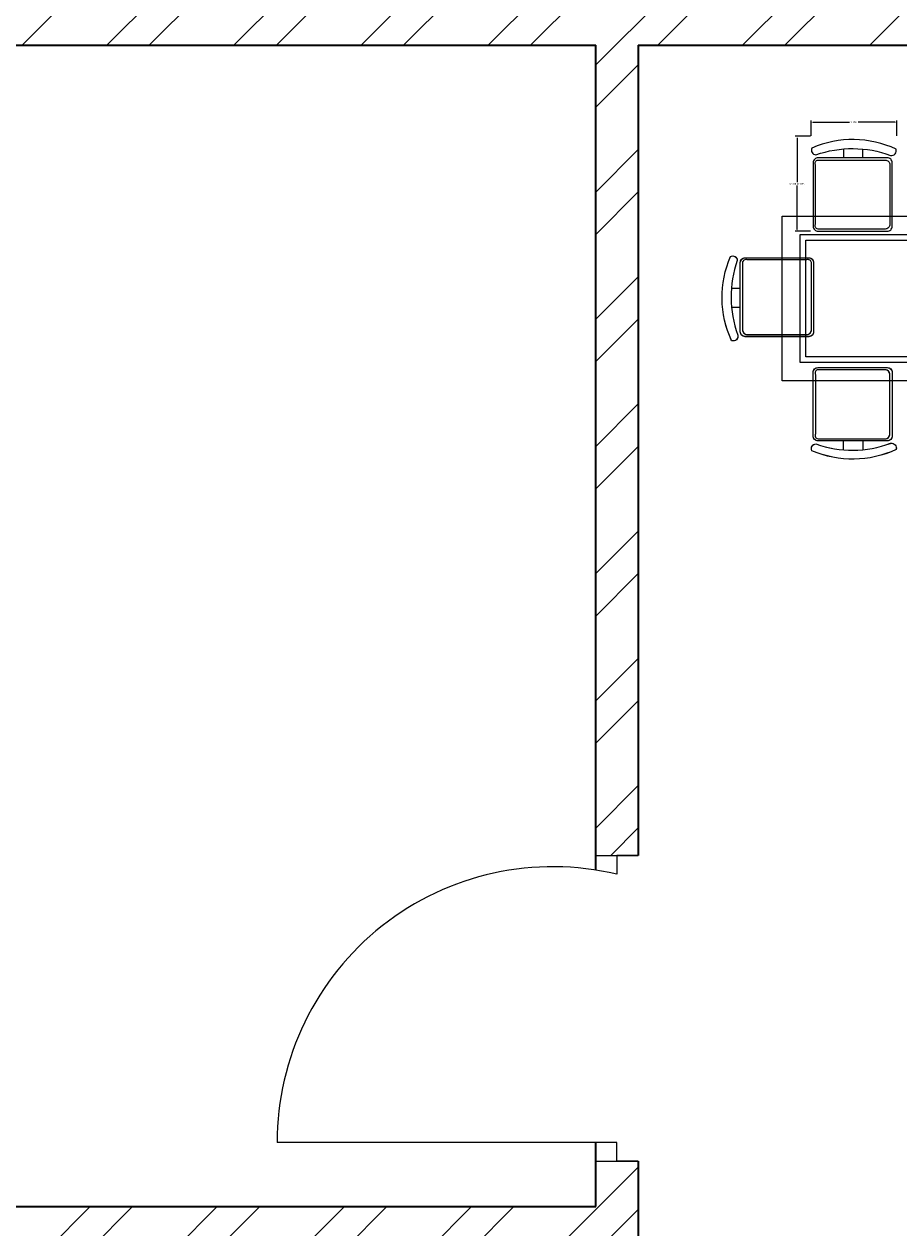
# Model space of a CAD drawing. Units: inches. Extents: x 2120 to 4013, y 1390 to 3019.
# Tile 6 of 59: x 2355 to 2448, y 1740 to 1868. Entities that reach past the tile are written whole.
import ezdxf

# ---------------------------------------------------------------- set-up
doc = ezdxf.new("R2010")
doc.units = ezdxf.units.IN
for name, color, linetype, lineweight in [('A-ANNO-DIMS', 2, 'Continuous', 18), ('A-DOOR', 3, 'Continuous', 18), ('A-FURN', 8, 'Continuous', 13), ('A-WALL', 7, 'Continuous', 35), ('A-WALL-PATT', 252, 'Continuous', 13)]:
    doc.layers.add(name, color=color, linetype=linetype, lineweight=lineweight)
doc.styles.get("Standard").update_dxf_attribs({"font": 'arial.ttf'})
doc.dimstyles.get("Standard").update_dxf_attribs({"dimtxt": 0.18, "dimasz": 0.18, "dimexe": 0.18, "dimexo": 0.0625, "dimgap": 0.09, "dimtad": 0, "dimtih": 1, "dimtoh": 1, "dimdec": 4, "dimzin": 0, "dimdsep": 46, "dimtxsty": 'Standard', "dimcen": 0.09, "dimadec": 0, "dimazin": 0, "dimtfac": 1, "dimtdec": 4, "dimtofl": 0, "dimtmove": 0, "dimatfit": 3, "dimfxl": 1, "dimtolj": 1, "dimtzin": 0, "dimarcsym": 0})

# ---------------------------------------------------------------- blocks, each defined once
blk = doc.blocks.new('DOOR-SWING-36IN-103p48DEG')
for p, q in [((33.75, 32.39), (38.25, 32.39)), ((38.25, 32.39), (36, 32.39)), ((36, 32.39), (36, 30.39)), ((36, 2), (0, 2)), ((36, 0), (36, 2)), ((33.75, 0), (38.25, 0)), ((38.25, 0), (36, 0))]:
    blk.add_line(p, q)
blk.add_arc((29.19, 2), 29.19, 76.5207, 180)
blk = doc.blocks.new('TABLE-DINING')
for points in [[(0, 17.41), (29.01, 17.41), (29.01, 0), (0, 0)], [(1.93, 15.47), (27.08, 15.47), (27.08, 1.93), (1.93, 1.93)], [(2.51, 14.89), (26.5, 14.89), (26.5, 2.51), (2.51, 2.51)]]:
    blk.add_lwpolyline(points, close=True)
blk = doc.blocks.new('CHAIR-DINING-07')
for points in [[(0.62, 8.03, -0.578392), (0.02, 8.69, -0.214524), (8.94, 8.81, -0.552014), (8.52, 8.09, 0.175809), (0.62, 8.03)], [(8.29, 7.77, -0.414214), (8.81, 7.26), (8.81, 0.51, -0.414214), (8.29, 0), (0.96, 0, -0.414214), (0.45, 0.51), (0.45, 7.26, -0.414214), (0.96, 7.77), (8.29, 7.77)], [(3.54, 7.77), (3.54, 8.7, 0.064759)]]:
    blk.add_lwpolyline(points, format="xyb")
blk.add_lwpolyline([(5.59, 8.72), (5.59, 7.77)])
blk.add_lwpolyline([(8.29, 7.54), (1.19, 7.54, 0.414214), (0.68, 7.03), (0.68, 0.74, 0.414214), (1.19, 0.23), (8.29, 0.23, 0.512069), (8.58, 0.74), (8.58, 7.03, 0.512069)], format="xyb", close=True)
blk = doc.blocks.new('CHAIR-DINING-08')
for points in [[(0.47, 8.09, -0.175809), (8.38, 8.03, 0.578392), (8.97, 8.69, 0.214524), (0.06, 8.81, 0.552014), (0.47, 8.09, -0.065079)], [(8.04, 7.77), (0.71, 7.77, 0.414214), (0.19, 7.26), (0.19, 0.51, 0.414214), (0.71, 0), (8.04, 0, 0.414214), (8.55, 0.51), (8.55, 7.26, 0.414214), (8.04, 7.77)], [(5.46, 7.77), (5.46, 8.7, -0.064759)]]:
    blk.add_lwpolyline(points, format="xyb")
blk.add_lwpolyline([(3.41, 8.72), (3.41, 7.77)])
blk.add_lwpolyline([(0.71, 7.54), (7.81, 7.54, -0.414214), (8.32, 7.03), (8.32, 0.74, -0.414214), (7.81, 0.23), (0.71, 0.23, -0.512069), (0.42, 0.74), (0.42, 7.03, -0.512069)], format="xyb", close=True)
blk = doc.blocks.new('CHAIR-DINING-11')
for points in [[(0.47, 8.09, -0.175809), (8.38, 8.03, 0.578392), (8.97, 8.69, 0.214524), (0.06, 8.81, 0.552014), (0.47, 8.09, -0.065079)], [(8.04, 7.77), (0.71, 7.77, 0.414214), (0.19, 7.26), (0.19, 0.51, 0.414214), (0.71, 0), (8.04, 0, 0.414214), (8.55, 0.51), (8.55, 7.26, 0.414214), (8.04, 7.77)], [(5.46, 7.77), (5.46, 8.7, -0.064759)]]:
    blk.add_lwpolyline(points, format="xyb")
blk.add_lwpolyline([(3.41, 8.72), (3.41, 7.77)])
blk.add_lwpolyline([(0.71, 7.54), (7.81, 7.54, -0.414214), (8.32, 7.03), (8.32, 0.74, -0.414214), (7.81, 0.23), (0.71, 0.23, -0.512069), (0.42, 0.74), (0.42, 7.03, -0.512069)], format="xyb", close=True)
blk = doc.blocks.new('CHAIR-DINING-16')
for points in [[(8.04, 1.93), (0.71, 1.93, -0.414214), (0.19, 2.45), (0.19, 9.19, -0.414214), (0.71, 9.7), (8.04, 9.7, -0.414214), (8.55, 9.19), (8.55, 2.45, -0.414214), (8.04, 1.93)], [(8.38, 1.68, -0.578392), (8.97, 1.02, -0.214524), (0.06, 0.9, -0.552014), (0.47, 1.62, 0.175809), (8.38, 1.68)], [(5.46, 1.93), (5.46, 1.01, 0.064759)]]:
    blk.add_lwpolyline(points, format="xyb")
blk.add_lwpolyline([(0.71, 2.16), (7.81, 2.16, 0.414214), (8.32, 2.68), (8.32, 8.96, 0.414214), (7.81, 9.47), (0.71, 9.47, 0.512069), (0.42, 8.96), (0.42, 2.68, 0.512069)], format="xyb", close=True)
blk.add_lwpolyline([(3.41, 0.99), (3.41, 1.93)])
blk = doc.blocks.new('*D101')
at = {"layer": 'A-ANNO-DIMS', "color": 0, "lineweight": -2, "transparency": 16777216}
for p, q in [((2438.5, 1855.88), (2436.88, 1855.88)), ((2437.06, 1855.7), (2437.06, 1851.04)), ((2437.06, 1846.01), (2437.06, 1850.67)), ((2438.5, 1845.83), (2436.88, 1845.83))]:
    blk.add_line(p, q, dxfattribs=at)
at = {"layer": 'A-ANNO-DIMS', "color": 0, "transparency": 16777216}
for points in [[(2437.03, 1855.7), (2437.09, 1855.7), (2437.06, 1855.88)], [(2437.03, 1846.01), (2437.09, 1846.01), (2437.06, 1845.83)]]:
    blk.add_solid(points, dxfattribs=at)
at = {"layer": 'Defpoints', "color": 0, "transparency": 16777216}
for p in [(2437.06, 1855.88), (2438.56, 1855.88), (2438.56, 1845.83)]:
    blk.add_point(p, dxfattribs=at)
at = {"layer": 'A-ANNO-DIMS', "color": 0, "transparency": 16777216, "insert": (2437.06, 1850.85), "char_height": 0.18, "attachment_point": 5}
blk.add_mtext('\\A1;CHAIR 10 TYP.', dxfattribs=at)
blk = doc.blocks.new('*D102')
at = {"layer": 'A-ANNO-DIMS', "color": 0, "lineweight": -2, "transparency": 16777216}
for p, q in [((2438.56, 1855.94), (2438.56, 1857.56)), ((2438.74, 1857.38), (2442.63, 1857.38)), ((2447.44, 1857.38), (2443.55, 1857.38)), ((2447.62, 1855.94), (2447.62, 1857.56))]:
    blk.add_line(p, q, dxfattribs=at)
at = {"layer": 'A-ANNO-DIMS', "color": 0, "transparency": 16777216}
for points in [[(2438.74, 1857.41), (2438.74, 1857.35), (2438.56, 1857.38)], [(2447.44, 1857.41), (2447.44, 1857.35), (2447.62, 1857.38)]]:
    blk.add_solid(points, dxfattribs=at)
at = {"layer": 'Defpoints', "color": 0, "transparency": 16777216}
for p in [(2447.62, 1857.38), (2438.56, 1855.88), (2447.62, 1855.88)]:
    blk.add_point(p, dxfattribs=at)
at = {"layer": 'A-ANNO-DIMS', "color": 0, "transparency": 16777216, "insert": (2443.09, 1857.38), "char_height": 0.18, "attachment_point": 5}
blk.add_mtext('\\A1;9 TYP.', dxfattribs=at)

msp = doc.modelspace()

# ---------------------------------------------------------------- hatches: boundary and pattern name
at = {"layer": 'A-WALL-PATT'}
h = msp.add_hatch(dxfattribs=at)
h.set_pattern_fill('ANSI32', color=256)
h.paths.add_polyline_path([(2271.7331, 2343.531), (2283.3788, 2343.531), (2283.3788, 2348.031), (2283.3788, 2352.5306), (2262.7331, 2352.5306), (2262.7331, 2182.638), (2267.2331, 2182.638), (2271.7331, 2182.638), (2271.7331, 2219.031), (2391.7331, 2219.031), (2391.7331, 2214.189), (2393.9831, 2214.189), (2396.2331, 2214.189), (2396.2331, 2219.031), (2420.2331, 2219.031), (2420.2331, 2225.7535), (2417.2197, 2225.7535), (2415.7331, 2225.7535), (2415.7331, 2223.5306), (2271.7331, 2223.5306)])
h.paths.add_polyline_path([(2380.0942, 2352.5306), (2343.3788, 2352.5306), (2343.3788, 2343.531), (2363.2331, 2343.531), (2363.2331, 2288.8489), (2365.4831, 2288.8489), (2367.7331, 2288.8489), (2367.7331, 2343.531), (2380.0942, 2343.531)], flags=17)
h.paths.add_polyline_path([(2432.4339, 2352.5306), (2404.0943, 2352.5306), (2404.0943, 2343.531), (2415.7331, 2343.531), (2415.7331, 2264.0306), (2367.7331, 2264.0306), (2367.7331, 2266.4872), (2363.2331, 2266.4872), (2363.2331, 2259.531), (2367.7331, 2259.531), (2415.7331, 2259.531), (2415.7331, 2255.0658), (2420.2331, 2255.0658), (2420.2331, 2259.531), (2424.5717, 2259.531), (2424.5717, 2261.781), (2424.5717, 2264.0306), (2420.2331, 2264.0306), (2420.2331, 2343.531), (2432.4339, 2343.531)])
h.paths.add_polyline_path([(2508.9115, 2352.5306), (2456.4339, 2352.5306), (2456.4339, 2343.531), (2468.2331, 2343.531), (2468.2331, 2264.0306), (2448.0487, 2264.0306), (2448.0487, 2259.531), (2468.2331, 2259.531), (2468.2331, 2255.5496), (2472.7331, 2255.5496), (2472.7331, 2343.531), (2508.9115, 2343.531)])
h.paths.add_polyline_path([(2637.7331, 2352.5306), (2544.9116, 2352.5306), (2544.9116, 2343.531), (2589.7331, 2343.531), (2633.2331, 2343.531), (2637.7331, 2343.531)])
h.paths.add_polyline_path([(2594.2331, 2343.5306), (2589.7331, 2343.5306), (2589.7331, 2259.5306), (2589.7331, 2252.4915), (2591.9831, 2252.4915), (2594.2331, 2252.4915)])
h.paths.add_polyline_path([(2637.7331, 2223.5306), (2594.2331, 2223.5306), (2594.2331, 2230.1988), (2591.9831, 2230.1988), (2589.7331, 2230.1988), (2589.7331, 2223.5306), (2472.7331, 2223.5306), (2468.2331, 2223.5306), (2468.2331, 2219.031), (2628.7331, 2219.031), (2628.7331, 2138.031), (2637.7331, 2138.031)])
h.paths.add_polyline_path([(3822.6535, 2458.4402), (3874.9468, 2458.4402), (3874.9468, 2476.9866), (3822.6535, 2476.9866)], flags=9)
h.paths.add_polyline_path([(3834.6921, 2781.8174), (3935.9206, 2781.8174), (3935.9206, 2800.3638), (3834.6921, 2800.3638)], flags=9)
h.paths.add_polyline_path([(3832.2843, 2837.9683), (3884.5776, 2837.9683), (3884.5776, 2856.5146), (3832.2843, 2856.5146)], flags=9)
h.paths.add_polyline_path([(3830.9388, 2861.4782), (3956.8958, 2861.4782), (3956.8958, 2880.0245), (3830.9388, 2880.0245)], flags=9)
h.paths.add_polyline_path([(3870.6966, 2352.5752), (3887.9272, 2352.5752), (3887.9272, 2377.3037), (3870.6966, 2377.3037)], flags=9)
h.paths.add_polyline_path([(3289.2701, 2413.161), (3435.2223, 2413.161), (3435.2223, 2450.2538), (3289.2701, 2450.2538)], flags=9)
h.paths.add_polyline_path([(2487.6944, 2414.3601), (2637.8335, 2414.3601), (2637.8335, 2451.4528), (2487.6944, 2451.4528)], flags=9)
h.paths.add_polyline_path([(2567.3724, 1457.9199), (2815.296, 1457.9199), (2815.296, 1495.0127), (2567.3724, 1495.0127)], flags=9)
h.paths.add_polyline_path([(2655.3825, 2093.2363), (2685.9555, 2093.2363), (2685.9555, 2111.8937), (2655.3825, 2111.8937)], flags=9)
h.paths.add_polyline_path([(2543.9218, 1550.6671), (2587.8406, 1550.6671), (2587.8406, 1569.3244), (2543.9218, 1569.3244)], flags=9)
h.paths.add_polyline_path([(2905.1384, 1543.8113), (2949.0572, 1543.8113), (2949.0572, 1562.4686), (2905.1384, 1562.4686)], flags=9)
h.paths.add_polyline_path([(2736.4118, 1702.4736), (2784.2153, 1702.4736), (2784.2153, 1721.1309), (2736.4118, 1721.1309)], flags=9)
h.paths.add_polyline_path([(2912.8666, 1710.4168), (2951.707, 1710.4168), (2951.707, 1729.0741), (2912.8666, 1729.0741)], flags=9)
h.paths.add_polyline_path([(2923.5785, 1763.5038), (2959.7279, 1763.5038), (2959.7279, 1782.1611), (2923.5785, 1782.1611)], flags=9)
h.paths.add_polyline_path([(2925.2114, 1809.6137), (2967.1861, 1809.6137), (2967.1861, 1828.271), (2925.2114, 1828.271)], flags=9)
h.paths.add_polyline_path([(2996.2711, 1878.9003), (2996.2711, 1913.109), (2977.6138, 1913.109), (2977.6138, 1878.9003)], flags=9)
h.paths.add_polyline_path([(2883.0859, 1895.7192), (2927.1855, 1895.7192), (2927.1855, 1914.3766), (2883.0859, 1914.3766)], flags=9)
h.paths.add_polyline_path([(2787.3924, 1810.8013), (2841.0213, 1810.8013), (2841.0213, 1829.4587), (2787.3924, 1829.4587)], flags=9)
h.paths.add_polyline_path([(2775.6399, 2101.7395), (2829.2689, 2101.7395), (2829.2689, 2120.3968), (2775.6399, 2120.3968)], flags=9)
h.paths.add_polyline_path([(2913.0263, 2075.817), (2951.8667, 2075.817), (2951.8667, 2094.4744), (2913.0263, 2094.4744)], flags=9)
h.paths.add_polyline_path([(2929.966, 2133.3669), (2966.1154, 2133.3669), (2966.1154, 2152.0243), (2929.966, 2152.0243)], flags=9)
h.paths.add_polyline_path([(2932.7502, 2182.6088), (2968.8996, 2182.6088), (2968.8996, 2201.2662), (2932.7502, 2201.2662)], flags=9)
h.paths.add_polyline_path([(2996.0681, 2266.3173), (2996.0681, 2300.5261), (2977.4108, 2300.5261), (2977.4108, 2266.3173)], flags=9)
h.paths.add_polyline_path([(2885.1039, 2279.2186), (2929.2035, 2279.2186), (2929.2035, 2297.8759), (2885.1039, 2297.8759)], flags=9)
h.paths.add_polyline_path([(2735.7042, 2218.3197), (2783.5078, 2218.3197), (2783.5078, 2236.9771), (2735.7042, 2236.9771)], flags=9)
h.paths.add_polyline_path([(2635.6049, 2044.0085), (2648.9678, 2044.0085), (2648.9678, 2054.312), (2635.6049, 2054.312)], flags=9)
h.paths.add_polyline_path([(2714.0148, 1923.0473), (2727.3777, 1923.0473), (2727.3777, 1933.3508), (2714.0148, 1933.3508)], flags=9)
h.paths.add_polyline_path([(2709.0345, 1988.1628), (2722.3974, 1988.1628), (2722.3974, 1998.4663), (2709.0345, 1998.4663)], flags=9)
h.paths.add_polyline_path([(2592.8935, 1962.1763), (2606.2564, 1962.1763), (2606.2564, 1972.4799), (2592.8935, 1972.4799)], flags=9)
h.paths.add_polyline_path([(2618.3996, 1985.9724), (2644.1942, 1985.9724), (2644.1942, 1996.2759), (2618.3996, 1996.2759)], flags=9)
h.paths.add_polyline_path([(2601.279, 1920.5869), (2614.6419, 1920.5869), (2614.6419, 1930.8904), (2601.279, 1930.8904)], flags=9)
h.paths.add_polyline_path([(2692.3278, 1932.7645), (2704.5311, 1932.7645), (2704.5311, 1943.0681), (2692.3278, 1943.0681)], flags=9)
h.paths.add_polyline_path([(2311.122, 1672.7318), (2355.0408, 1672.7318), (2355.0408, 1691.3892), (2311.122, 1691.3892)], flags=9)
h.paths.add_polyline_path([(2456.2551, 1632.3198), (2492.4796, 1632.3198), (2492.4796, 1650.9772), (2456.2551, 1650.9772)], flags=9)
h.paths.add_polyline_path([(2401.0766, 1631.4793), (2437.301, 1631.4793), (2437.301, 1650.1367), (2401.0766, 1650.1367)], flags=9)
h.paths.add_polyline_path([(2546.7054, 1700.9235), (2594.509, 1700.9235), (2594.509, 1719.5809), (2546.7054, 1719.5809)], flags=9)
h.paths.add_polyline_path([(2445.4866, 1766.9937), (2497.5261, 1766.9937), (2497.5261, 1785.651), (2445.4866, 1785.651)], flags=9)
h.paths.add_polyline_path([(2287.9992, 1739.7675), (2326.8396, 1739.7675), (2326.8396, 1758.4248), (2287.9992, 1758.4248)], flags=9)
h.paths.add_polyline_path([(2458.5279, 1924.7607), (2510.5675, 1924.7607), (2510.5675, 1943.4181), (2458.5279, 1943.4181)], flags=9)
h.paths.add_polyline_path([(2309.2811, 1902.7642), (2345.4305, 1902.7642), (2345.4305, 1921.4215), (2309.2811, 1921.4215)], flags=9)
h.paths.add_polyline_path([(2490.7554, 2018.9392), (2530.7896, 2018.9392), (2530.7896, 2037.5965), (2490.7554, 2037.5965)], flags=9)
h.paths.add_polyline_path([(2402.143, 2024.7393), (2438.5414, 2024.7393), (2438.5414, 2043.3966), (2402.143, 2043.3966)], flags=9)
h.paths.add_polyline_path([(2287.856, 1931.7926), (2326.6964, 1931.7926), (2326.6964, 1950.4499), (2287.856, 1950.4499)], flags=9)
h.paths.add_polyline_path([(2281.7979, 2193.5771), (2320.6383, 2193.5771), (2320.6383, 2212.2344), (2281.7979, 2212.2344)], flags=25)
h.paths.add_polyline_path([(2484.0754, 2093.892), (2536.115, 2093.892), (2536.115, 2112.5494), (2484.0754, 2112.5494)], flags=9)
h.paths.add_polyline_path([(2624.7948, 2281.8639), (2624.7948, 2311.4137), (2606.1375, 2311.4137), (2606.1375, 2281.8639)], flags=9)
h.paths.add_polyline_path([(2507.5036, 2290.3639), (2541.934, 2290.3639), (2541.934, 2309.0212), (2507.5036, 2309.0212)], flags=9)
h.paths.add_polyline_path([(2423.1076, 2285.2202), (2459.332, 2285.2202), (2459.332, 2303.8776), (2423.1076, 2303.8776)], flags=9)
h.paths.add_polyline_path([(2374.5467, 2289.6272), (2410.7711, 2289.6272), (2410.7711, 2308.2846), (2374.5467, 2308.2846)], flags=25)
h.paths.add_polyline_path([(2277.4907, 2227.5651), (2316.3311, 2227.5651), (2316.3311, 2246.2224), (2277.4907, 2246.2224)], flags=25)
h.paths.add_polyline_path([(2655.3825, 2093.2367), (2685.9555, 2093.2367), (2685.9555, 2111.894), (2655.3825, 2111.894)], flags=9)
h.paths.add_polyline_path([(2543.9217, 1550.6674), (2587.8406, 1550.6674), (2587.8406, 1569.3247), (2543.9217, 1569.3247)], flags=9)
h.paths.add_polyline_path([(2905.1384, 1543.8116), (2949.0572, 1543.8116), (2949.0572, 1562.4689), (2905.1384, 1562.4689)], flags=9)
h.paths.add_polyline_path([(2736.4118, 1702.4739), (2784.2153, 1702.4739), (2784.2153, 1721.1312), (2736.4118, 1721.1312)], flags=9)
h.paths.add_polyline_path([(2912.8666, 1710.4171), (2951.707, 1710.4171), (2951.707, 1729.0744), (2912.8666, 1729.0744)], flags=9)
h.paths.add_polyline_path([(2923.5785, 1763.5041), (2959.7279, 1763.5041), (2959.7279, 1782.1614), (2923.5785, 1782.1614)], flags=9)
h.paths.add_polyline_path([(2925.2114, 1809.614), (2967.1861, 1809.614), (2967.1861, 1828.2713), (2925.2114, 1828.2713)], flags=9)
h.paths.add_polyline_path([(2996.2711, 1878.9006), (2996.2711, 1913.1094), (2977.6137, 1913.1094), (2977.6137, 1878.9006)], flags=9)
h.paths.add_polyline_path([(2883.0859, 1895.7195), (2927.1855, 1895.7195), (2927.1855, 1914.3769), (2883.0859, 1914.3769)], flags=9)
h.paths.add_polyline_path([(2787.3924, 1810.8016), (2841.0213, 1810.8016), (2841.0213, 1829.459), (2787.3924, 1829.459)], flags=9)
h.paths.add_polyline_path([(2775.6399, 2101.7398), (2829.2688, 2101.7398), (2829.2688, 2120.3971), (2775.6399, 2120.3971)], flags=9)
h.paths.add_polyline_path([(2913.0263, 2075.8173), (2951.8667, 2075.8173), (2951.8667, 2094.4747), (2913.0263, 2094.4747)], flags=9)
h.paths.add_polyline_path([(2929.966, 2133.3672), (2966.1154, 2133.3672), (2966.1154, 2152.0246), (2929.966, 2152.0246)], flags=9)
h.paths.add_polyline_path([(2932.7502, 2182.6091), (2968.8996, 2182.6091), (2968.8996, 2201.2665), (2932.7502, 2201.2665)], flags=9)
h.paths.add_polyline_path([(2996.0681, 2266.3176), (2996.0681, 2300.5264), (2977.4108, 2300.5264), (2977.4108, 2266.3176)], flags=9)
h.paths.add_polyline_path([(2885.1039, 2279.2189), (2929.2035, 2279.2189), (2929.2035, 2297.8762), (2885.1039, 2297.8762)], flags=9)
h.paths.add_polyline_path([(2735.7042, 2218.32), (2783.5078, 2218.32), (2783.5078, 2236.9774), (2735.7042, 2236.9774)], flags=9)
h.paths.add_polyline_path([(2635.6048, 2044.0088), (2648.9677, 2044.0088), (2648.9677, 2054.3123), (2635.6048, 2054.3123)], flags=9)
h.paths.add_polyline_path([(2714.0148, 1923.0476), (2727.3777, 1923.0476), (2727.3777, 1933.3511), (2714.0148, 1933.3511)], flags=9)
h.paths.add_polyline_path([(2709.0345, 1988.1631), (2722.3974, 1988.1631), (2722.3974, 1998.4666), (2709.0345, 1998.4666)], flags=9)
h.paths.add_polyline_path([(2592.8935, 1962.1766), (2606.2564, 1962.1766), (2606.2564, 1972.4802), (2592.8935, 1972.4802)], flags=9)
h.paths.add_polyline_path([(2618.3995, 1985.9727), (2644.1942, 1985.9727), (2644.1942, 1996.2762), (2618.3995, 1996.2762)], flags=9)
h.paths.add_polyline_path([(2601.279, 1920.5872), (2614.6419, 1920.5872), (2614.6419, 1930.8908), (2601.279, 1930.8908)], flags=9)
h.paths.add_polyline_path([(2692.3278, 1932.7648), (2704.5311, 1932.7648), (2704.5311, 1943.0684), (2692.3278, 1943.0684)], flags=9)
h.paths.add_polyline_path([(2311.122, 1672.7321), (2355.0408, 1672.7321), (2355.0408, 1691.3895), (2311.122, 1691.3895)], flags=9)
h.paths.add_polyline_path([(2456.2551, 1632.3201), (2492.4795, 1632.3201), (2492.4795, 1650.9775), (2456.2551, 1650.9775)], flags=9)
h.paths.add_polyline_path([(2401.0766, 1631.4796), (2437.301, 1631.4796), (2437.301, 1650.137), (2401.0766, 1650.137)], flags=9)
h.paths.add_polyline_path([(2546.7054, 1700.9238), (2594.509, 1700.9238), (2594.509, 1719.5812), (2546.7054, 1719.5812)], flags=9)
h.paths.add_polyline_path([(2445.4866, 1766.994), (2497.5261, 1766.994), (2497.5261, 1785.6513), (2445.4866, 1785.6513)], flags=9)
h.paths.add_polyline_path([(2287.9992, 1739.7678), (2326.8396, 1739.7678), (2326.8396, 1758.4251), (2287.9992, 1758.4251)], flags=9)
h.paths.add_polyline_path([(2458.5279, 1924.7611), (2510.5675, 1924.7611), (2510.5675, 1943.4184), (2458.5279, 1943.4184)], flags=9)
h.paths.add_polyline_path([(2309.2811, 1902.7645), (2345.4305, 1902.7645), (2345.4305, 1921.4218), (2309.2811, 1921.4218)], flags=9)
h.paths.add_polyline_path([(2490.7554, 2018.9395), (2530.7895, 2018.9395), (2530.7895, 2037.5968), (2490.7554, 2037.5968)], flags=9)
h.paths.add_polyline_path([(2402.143, 2024.7396), (2438.5413, 2024.7396), (2438.5413, 2043.3969), (2402.143, 2043.3969)], flags=9)
h.paths.add_polyline_path([(2287.856, 1931.7929), (2326.6964, 1931.7929), (2326.6964, 1950.4502), (2287.856, 1950.4502)], flags=9)
h.paths.add_polyline_path([(2281.7979, 2193.5774), (2320.6383, 2193.5774), (2320.6383, 2212.2347), (2281.7979, 2212.2347)], flags=25)
h.paths.add_polyline_path([(2484.0754, 2093.8924), (2536.115, 2093.8924), (2536.115, 2112.5497), (2484.0754, 2112.5497)], flags=9)
h.paths.add_polyline_path([(2624.7948, 2281.8642), (2624.7948, 2311.414), (2606.1374, 2311.414), (2606.1374, 2281.8642)], flags=9)
h.paths.add_polyline_path([(2507.5035, 2290.3642), (2541.934, 2290.3642), (2541.934, 2309.0215), (2507.5035, 2309.0215)], flags=9)
h.paths.add_polyline_path([(2423.1075, 2285.2205), (2459.332, 2285.2205), (2459.332, 2303.8779), (2423.1075, 2303.8779)], flags=9)
h.paths.add_polyline_path([(2374.5467, 2289.6275), (2410.7711, 2289.6275), (2410.7711, 2308.2849), (2374.5467, 2308.2849)], flags=25)
h.paths.add_polyline_path([(2277.4907, 2227.5654), (2316.3311, 2227.5654), (2316.3311, 2246.2227), (2277.4907, 2246.2227)], flags=25)
h = msp.add_hatch(dxfattribs=at)
h.set_pattern_fill('ANSI32', color=256)
h.paths.add_polyline_path([(2271.7331, 1980.389), (2262.7331, 1980.389), (2262.7331, 1912.8434), (2267.2331, 1912.8434), (2271.7331, 1912.8434), (2271.7331, 1922.531), (2351.2331, 1922.531), (2351.2331, 1901.4728), (2355.7331, 1901.4728), (2355.7331, 1922.531), (2357.9815, 1922.531), (2357.9815, 1926.5306), (2271.7331, 1926.5306)])
h.paths.add_polyline_path([(2589.2331, 1949.1622), (2584.7331, 1949.1622), (2580.2331, 1949.1622), (2580.2331, 1874.5306), (2355.7331, 1874.5306), (2355.7331, 1880.1922), (2351.2331, 1880.1922), (2351.2331, 1874.5306), (2271.7331, 1874.5306), (2271.7331, 1888.8431), (2262.7331, 1888.8431), (2262.7331, 1842.2909), (2267.2331, 1842.2909), (2271.7331, 1842.2909), (2271.7331, 1865.531), (2415.7331, 1865.531), (2415.7331, 1779.7286), (2420.2331, 1779.7286), (2420.2331, 1865.531), (2589.2331, 1865.531)])
h.paths.add_polyline_path([(2271.7331, 1782.2906), (2262.7331, 1782.2906), (2262.7331, 1711.4639), (2267.2331, 1711.4639), (2271.7331, 1711.4639), (2271.7331, 1738.031), (2420.2331, 1738.031), (2420.2331, 1742.531), (2420.2331, 1747.3376), (2417.9831, 1747.3376), (2415.7331, 1747.3376), (2415.7331, 1742.5306), (2271.7331, 1742.5306)])
h.paths.add_polyline_path([(2271.7331, 1627.031), (2362.3957, 1627.031), (2362.3957, 1629.281), (2362.3957, 1631.5306), (2271.7331, 1631.5306), (2271.7331, 1675.4636), (2262.7331, 1675.4636), (2262.7331, 1581.531), (2405.3032, 1581.531), (2405.3032, 1586.031), (2405.3032, 1590.5306), (2396.2331, 1590.5306), (2396.2331, 1691.4513), (2418.7206, 1691.4513), (2418.7206, 1695.951), (2396.2331, 1695.951), (2391.7331, 1695.951), (2391.7331, 1631.5306), (2386.7425, 1631.5306), (2386.7425, 1629.2806), (2386.7425, 1627.031), (2391.7331, 1627.031), (2391.7331, 1586.1709), (2271.7331, 1586.1709)])
h.paths.add_polyline_path([(2459.6703, 1590.5306), (2429.3032, 1590.5306), (2429.3032, 1581.531), (2459.6703, 1581.531), (2459.6703, 1586.031)])
h.paths.add_polyline_path([(2501.2331, 1590.531), (2501.2331, 1665.0195), (2498.9831, 1665.0195), (2496.7331, 1665.0195), (2496.7331, 1590.5306), (2483.8201, 1590.5306), (2483.8201, 1590.1579), (2483.6704, 1590.1579), (2483.6704, 1581.531), (2505.0196, 1581.531), (2505.0196, 1583.781), (2505.0196, 1586.0306), (2501.2331, 1586.0306)])
h.paths.add_polyline_path([(2544.1361, 1583.781), (2544.1361, 1586.0306), (2527.1368, 1586.0306), (2527.1368, 1583.7806), (2527.1368, 1581.531), (2544.1361, 1581.531)])
h.paths.add_polyline_path([(3822.6535, 2458.4402), (3874.9468, 2458.4402), (3874.9468, 2476.9866), (3822.6535, 2476.9866)], flags=9)
h.paths.add_polyline_path([(3834.6921, 2781.8174), (3935.9206, 2781.8174), (3935.9206, 2800.3638), (3834.6921, 2800.3638)], flags=9)
h.paths.add_polyline_path([(3832.2843, 2837.9683), (3884.5776, 2837.9683), (3884.5776, 2856.5146), (3832.2843, 2856.5146)], flags=9)
h.paths.add_polyline_path([(3830.9388, 2861.4782), (3956.8958, 2861.4782), (3956.8958, 2880.0245), (3830.9388, 2880.0245)], flags=9)
h.paths.add_polyline_path([(3870.6966, 2352.5752), (3887.9272, 2352.5752), (3887.9272, 2377.3037), (3870.6966, 2377.3037)], flags=9)
h.paths.add_polyline_path([(3289.2701, 2413.161), (3435.2223, 2413.161), (3435.2223, 2450.2538), (3289.2701, 2450.2538)], flags=9)
h.paths.add_polyline_path([(2487.6944, 2414.3601), (2637.8335, 2414.3601), (2637.8335, 2451.4528), (2487.6944, 2451.4528)], flags=9)
h.paths.add_polyline_path([(2567.3724, 1457.9199), (2815.296, 1457.9199), (2815.296, 1495.0127), (2567.3724, 1495.0127)], flags=9)
h.paths.add_polyline_path([(2655.3825, 2093.2363), (2685.9555, 2093.2363), (2685.9555, 2111.8937), (2655.3825, 2111.8937)], flags=9)
h.paths.add_polyline_path([(2543.9218, 1550.6671), (2587.8406, 1550.6671), (2587.8406, 1569.3244), (2543.9218, 1569.3244)], flags=9)
h.paths.add_polyline_path([(2905.1384, 1543.8113), (2949.0572, 1543.8113), (2949.0572, 1562.4686), (2905.1384, 1562.4686)], flags=9)
h.paths.add_polyline_path([(2736.4118, 1702.4736), (2784.2153, 1702.4736), (2784.2153, 1721.1309), (2736.4118, 1721.1309)], flags=9)
h.paths.add_polyline_path([(2912.8666, 1710.4168), (2951.707, 1710.4168), (2951.707, 1729.0741), (2912.8666, 1729.0741)], flags=9)
h.paths.add_polyline_path([(2923.5785, 1763.5038), (2959.7279, 1763.5038), (2959.7279, 1782.1611), (2923.5785, 1782.1611)], flags=9)
h.paths.add_polyline_path([(2925.2114, 1809.6137), (2967.1861, 1809.6137), (2967.1861, 1828.271), (2925.2114, 1828.271)], flags=9)
h.paths.add_polyline_path([(2996.2711, 1878.9003), (2996.2711, 1913.109), (2977.6138, 1913.109), (2977.6138, 1878.9003)], flags=9)
h.paths.add_polyline_path([(2883.0859, 1895.7192), (2927.1855, 1895.7192), (2927.1855, 1914.3766), (2883.0859, 1914.3766)], flags=9)
h.paths.add_polyline_path([(2787.3924, 1810.8013), (2841.0213, 1810.8013), (2841.0213, 1829.4587), (2787.3924, 1829.4587)], flags=9)
h.paths.add_polyline_path([(2775.6399, 2101.7395), (2829.2689, 2101.7395), (2829.2689, 2120.3968), (2775.6399, 2120.3968)], flags=9)
h.paths.add_polyline_path([(2913.0263, 2075.817), (2951.8667, 2075.817), (2951.8667, 2094.4744), (2913.0263, 2094.4744)], flags=9)
h.paths.add_polyline_path([(2929.966, 2133.3669), (2966.1154, 2133.3669), (2966.1154, 2152.0243), (2929.966, 2152.0243)], flags=9)
h.paths.add_polyline_path([(2932.7502, 2182.6088), (2968.8996, 2182.6088), (2968.8996, 2201.2662), (2932.7502, 2201.2662)], flags=9)
h.paths.add_polyline_path([(2996.0681, 2266.3173), (2996.0681, 2300.5261), (2977.4108, 2300.5261), (2977.4108, 2266.3173)], flags=9)
h.paths.add_polyline_path([(2885.1039, 2279.2186), (2929.2035, 2279.2186), (2929.2035, 2297.8759), (2885.1039, 2297.8759)], flags=9)
h.paths.add_polyline_path([(2735.7042, 2218.3197), (2783.5078, 2218.3197), (2783.5078, 2236.9771), (2735.7042, 2236.9771)], flags=9)
h.paths.add_polyline_path([(2635.6049, 2044.0085), (2648.9678, 2044.0085), (2648.9678, 2054.312), (2635.6049, 2054.312)], flags=9)
h.paths.add_polyline_path([(2714.0148, 1923.0473), (2727.3777, 1923.0473), (2727.3777, 1933.3508), (2714.0148, 1933.3508)], flags=9)
h.paths.add_polyline_path([(2709.0345, 1988.1628), (2722.3974, 1988.1628), (2722.3974, 1998.4663), (2709.0345, 1998.4663)], flags=9)
h.paths.add_polyline_path([(2592.8935, 1962.1763), (2606.2564, 1962.1763), (2606.2564, 1972.4799), (2592.8935, 1972.4799)], flags=9)
h.paths.add_polyline_path([(2618.3996, 1985.9724), (2644.1942, 1985.9724), (2644.1942, 1996.2759), (2618.3996, 1996.2759)], flags=9)
h.paths.add_polyline_path([(2601.279, 1920.5869), (2614.6419, 1920.5869), (2614.6419, 1930.8904), (2601.279, 1930.8904)], flags=9)
h.paths.add_polyline_path([(2692.3278, 1932.7645), (2704.5311, 1932.7645), (2704.5311, 1943.0681), (2692.3278, 1943.0681)], flags=9)
h.paths.add_polyline_path([(2311.122, 1672.7318), (2355.0408, 1672.7318), (2355.0408, 1691.3892), (2311.122, 1691.3892)], flags=25)
h.paths.add_polyline_path([(2456.2551, 1632.3198), (2492.4796, 1632.3198), (2492.4796, 1650.9772), (2456.2551, 1650.9772)], flags=9)
h.paths.add_polyline_path([(2401.0766, 1631.4793), (2437.301, 1631.4793), (2437.301, 1650.1367), (2401.0766, 1650.1367)], flags=9)
h.paths.add_polyline_path([(2546.7054, 1700.9235), (2594.509, 1700.9235), (2594.509, 1719.5809), (2546.7054, 1719.5809)], flags=9)
h.paths.add_polyline_path([(2445.4866, 1766.9937), (2497.5261, 1766.9937), (2497.5261, 1785.651), (2445.4866, 1785.651)], flags=9)
h.paths.add_polyline_path([(2287.9992, 1739.7675), (2326.8396, 1739.7675), (2326.8396, 1758.4248), (2287.9992, 1758.4248)], flags=24)
h.paths.add_polyline_path([(2458.5279, 1924.7607), (2510.5675, 1924.7607), (2510.5675, 1943.4181), (2458.5279, 1943.4181)], flags=25)
h.paths.add_polyline_path([(2309.2811, 1902.7642), (2345.4305, 1902.7642), (2345.4305, 1921.4215), (2309.2811, 1921.4215)], flags=25)
h.paths.add_polyline_path([(2490.7554, 2018.9392), (2530.7896, 2018.9392), (2530.7896, 2037.5965), (2490.7554, 2037.5965)], flags=9)
h.paths.add_polyline_path([(2402.143, 2024.7393), (2438.5414, 2024.7393), (2438.5414, 2043.3966), (2402.143, 2043.3966)], flags=9)
h.paths.add_polyline_path([(2287.856, 1931.7926), (2326.6964, 1931.7926), (2326.6964, 1950.4499), (2287.856, 1950.4499)], flags=25)
h.paths.add_polyline_path([(2281.7979, 2193.5771), (2320.6383, 2193.5771), (2320.6383, 2212.2344), (2281.7979, 2212.2344)], flags=9)
h.paths.add_polyline_path([(2484.0754, 2093.892), (2536.115, 2093.892), (2536.115, 2112.5494), (2484.0754, 2112.5494)], flags=9)
h.paths.add_polyline_path([(2624.7948, 2281.8639), (2624.7948, 2311.4137), (2606.1375, 2311.4137), (2606.1375, 2281.8639)], flags=9)
h.paths.add_polyline_path([(2507.5036, 2290.3639), (2541.934, 2290.3639), (2541.934, 2309.0212), (2507.5036, 2309.0212)], flags=9)
h.paths.add_polyline_path([(2423.1076, 2285.2202), (2459.332, 2285.2202), (2459.332, 2303.8776), (2423.1076, 2303.8776)], flags=9)
h.paths.add_polyline_path([(2374.5467, 2289.6272), (2410.7711, 2289.6272), (2410.7711, 2308.2846), (2374.5467, 2308.2846)], flags=9)
h.paths.add_polyline_path([(2277.4907, 2227.5651), (2316.3311, 2227.5651), (2316.3311, 2246.2224), (2277.4907, 2246.2224)], flags=9)
h.paths.add_polyline_path([(2655.3825, 2093.2367), (2685.9555, 2093.2367), (2685.9555, 2111.894), (2655.3825, 2111.894)], flags=9)
h.paths.add_polyline_path([(2543.9217, 1550.6674), (2587.8406, 1550.6674), (2587.8406, 1569.3247), (2543.9217, 1569.3247)], flags=9)
h.paths.add_polyline_path([(2905.1384, 1543.8116), (2949.0572, 1543.8116), (2949.0572, 1562.4689), (2905.1384, 1562.4689)], flags=9)
h.paths.add_polyline_path([(2736.4118, 1702.4739), (2784.2153, 1702.4739), (2784.2153, 1721.1312), (2736.4118, 1721.1312)], flags=9)
h.paths.add_polyline_path([(2912.8666, 1710.4171), (2951.707, 1710.4171), (2951.707, 1729.0744), (2912.8666, 1729.0744)], flags=9)
h.paths.add_polyline_path([(2923.5785, 1763.5041), (2959.7279, 1763.5041), (2959.7279, 1782.1614), (2923.5785, 1782.1614)], flags=9)
h.paths.add_polyline_path([(2925.2114, 1809.614), (2967.1861, 1809.614), (2967.1861, 1828.2713), (2925.2114, 1828.2713)], flags=9)
h.paths.add_polyline_path([(2996.2711, 1878.9006), (2996.2711, 1913.1094), (2977.6137, 1913.1094), (2977.6137, 1878.9006)], flags=9)
h.paths.add_polyline_path([(2883.0859, 1895.7195), (2927.1855, 1895.7195), (2927.1855, 1914.3769), (2883.0859, 1914.3769)], flags=9)
h.paths.add_polyline_path([(2787.3924, 1810.8016), (2841.0213, 1810.8016), (2841.0213, 1829.459), (2787.3924, 1829.459)], flags=9)
h.paths.add_polyline_path([(2775.6399, 2101.7398), (2829.2688, 2101.7398), (2829.2688, 2120.3971), (2775.6399, 2120.3971)], flags=9)
h.paths.add_polyline_path([(2913.0263, 2075.8173), (2951.8667, 2075.8173), (2951.8667, 2094.4747), (2913.0263, 2094.4747)], flags=9)
h.paths.add_polyline_path([(2929.966, 2133.3672), (2966.1154, 2133.3672), (2966.1154, 2152.0246), (2929.966, 2152.0246)], flags=9)
h.paths.add_polyline_path([(2932.7502, 2182.6091), (2968.8996, 2182.6091), (2968.8996, 2201.2665), (2932.7502, 2201.2665)], flags=9)
h.paths.add_polyline_path([(2996.0681, 2266.3176), (2996.0681, 2300.5264), (2977.4108, 2300.5264), (2977.4108, 2266.3176)], flags=9)
h.paths.add_polyline_path([(2885.1039, 2279.2189), (2929.2035, 2279.2189), (2929.2035, 2297.8762), (2885.1039, 2297.8762)], flags=9)
h.paths.add_polyline_path([(2735.7042, 2218.32), (2783.5078, 2218.32), (2783.5078, 2236.9774), (2735.7042, 2236.9774)], flags=9)
h.paths.add_polyline_path([(2635.6048, 2044.0088), (2648.9677, 2044.0088), (2648.9677, 2054.3123), (2635.6048, 2054.3123)], flags=9)
h.paths.add_polyline_path([(2714.0148, 1923.0476), (2727.3777, 1923.0476), (2727.3777, 1933.3511), (2714.0148, 1933.3511)], flags=9)
h.paths.add_polyline_path([(2709.0345, 1988.1631), (2722.3974, 1988.1631), (2722.3974, 1998.4666), (2709.0345, 1998.4666)], flags=9)
h.paths.add_polyline_path([(2592.8935, 1962.1766), (2606.2564, 1962.1766), (2606.2564, 1972.4802), (2592.8935, 1972.4802)], flags=9)
h.paths.add_polyline_path([(2618.3995, 1985.9727), (2644.1942, 1985.9727), (2644.1942, 1996.2762), (2618.3995, 1996.2762)], flags=9)
h.paths.add_polyline_path([(2601.279, 1920.5872), (2614.6419, 1920.5872), (2614.6419, 1930.8908), (2601.279, 1930.8908)], flags=9)
h.paths.add_polyline_path([(2692.3278, 1932.7648), (2704.5311, 1932.7648), (2704.5311, 1943.0684), (2692.3278, 1943.0684)], flags=9)
h.paths.add_polyline_path([(2311.122, 1672.7321), (2355.0408, 1672.7321), (2355.0408, 1691.3895), (2311.122, 1691.3895)], flags=25)
h.paths.add_polyline_path([(2456.2551, 1632.3201), (2492.4795, 1632.3201), (2492.4795, 1650.9775), (2456.2551, 1650.9775)], flags=9)
h.paths.add_polyline_path([(2401.0766, 1631.4796), (2437.301, 1631.4796), (2437.301, 1650.137), (2401.0766, 1650.137)], flags=9)
h.paths.add_polyline_path([(2546.7054, 1700.9238), (2594.509, 1700.9238), (2594.509, 1719.5812), (2546.7054, 1719.5812)], flags=9)
h.paths.add_polyline_path([(2445.4866, 1766.994), (2497.5261, 1766.994), (2497.5261, 1785.6513), (2445.4866, 1785.6513)], flags=9)
h.paths.add_polyline_path([(2287.9992, 1739.7678), (2326.8396, 1739.7678), (2326.8396, 1758.4251), (2287.9992, 1758.4251)], flags=24)
h.paths.add_polyline_path([(2458.5279, 1924.7611), (2510.5675, 1924.7611), (2510.5675, 1943.4184), (2458.5279, 1943.4184)], flags=25)
h.paths.add_polyline_path([(2309.2811, 1902.7645), (2345.4305, 1902.7645), (2345.4305, 1921.4218), (2309.2811, 1921.4218)], flags=25)
h.paths.add_polyline_path([(2490.7554, 2018.9395), (2530.7895, 2018.9395), (2530.7895, 2037.5968), (2490.7554, 2037.5968)], flags=9)
h.paths.add_polyline_path([(2402.143, 2024.7396), (2438.5413, 2024.7396), (2438.5413, 2043.3969), (2402.143, 2043.3969)], flags=9)
h.paths.add_polyline_path([(2287.856, 1931.7929), (2326.6964, 1931.7929), (2326.6964, 1950.4502), (2287.856, 1950.4502)], flags=25)
h.paths.add_polyline_path([(2281.7979, 2193.5774), (2320.6383, 2193.5774), (2320.6383, 2212.2347), (2281.7979, 2212.2347)], flags=9)
h.paths.add_polyline_path([(2484.0754, 2093.8924), (2536.115, 2093.8924), (2536.115, 2112.5497), (2484.0754, 2112.5497)], flags=9)
h.paths.add_polyline_path([(2624.7948, 2281.8642), (2624.7948, 2311.414), (2606.1374, 2311.414), (2606.1374, 2281.8642)], flags=9)
h.paths.add_polyline_path([(2507.5035, 2290.3642), (2541.934, 2290.3642), (2541.934, 2309.0215), (2507.5035, 2309.0215)], flags=9)
h.paths.add_polyline_path([(2423.1075, 2285.2205), (2459.332, 2285.2205), (2459.332, 2303.8779), (2423.1075, 2303.8779)], flags=9)
h.paths.add_polyline_path([(2374.5467, 2289.6275), (2410.7711, 2289.6275), (2410.7711, 2308.2849), (2374.5467, 2308.2849)], flags=9)
h.paths.add_polyline_path([(2277.4907, 2227.5654), (2316.3311, 2227.5654), (2316.3311, 2246.2227), (2277.4907, 2246.2227)], flags=9)

# ---------------------------------------------------------------- linework, layer by layer
at = {"layer": 'A-FURN'}
for points in [[(2430.7921, 1834.8388, -0.57839206), (2430.1339, 1834.2402, -0.21452438), (2430.0142, 1843.1595, -0.55201397), (2430.7323, 1842.7405, 0.17580937), (2430.7921, 1834.8388)], [(2431.0494, 1842.5097, -0.41421356), (2431.5626, 1843.0229), (2438.3077, 1843.0229, -0.41421356), (2438.8209, 1842.5097), (2438.8209, 1835.174, -0.41421356), (2438.3077, 1834.6608), (2431.5626, 1834.6608, -0.41421356), (2431.0494, 1835.174), (2431.0494, 1842.5097)], [(2431.0494, 1837.7507), (2430.1217, 1837.7507, 0.06475861)], [(2446.6253, 1823.6202), (2439.2896, 1823.6202, -0.41421356), (2438.7764, 1824.1334), (2438.7764, 1830.8784, -0.41421356), (2439.2896, 1831.3916), (2446.6253, 1831.3916, -0.41421356), (2447.1385, 1830.8784), (2447.1385, 1824.1334, -0.41421356), (2446.6253, 1823.6202)], [(2446.9605, 1823.3629, -0.57839206), (2447.5591, 1822.7046, -0.21452438), (2438.6398, 1822.585, -0.55201397), (2439.0588, 1823.303, 0.17580929), (2446.9605, 1823.3629)], [(2444.0486, 1823.6202), (2444.0486, 1822.6924, 0.06475861)]]:
    msp.add_lwpolyline(points, format="xyb", dxfattribs=at)
for points in [[(2431.2806, 1842.5066), (2431.2806, 1835.4052, 0.41421356), (2431.7939, 1834.892), (2438.0765, 1834.892, 0.41421356), (2438.5897, 1835.4052), (2438.5897, 1842.5066, 0.51206948), (2438.0765, 1842.7917), (2431.7939, 1842.7917, 0.51206948)], [(2439.2927, 1823.8514), (2446.3941, 1823.8514, 0.41421356), (2446.9073, 1824.3646), (2446.9073, 1830.6472, 0.41421356), (2446.3941, 1831.1604), (2439.2927, 1831.1604, 0.51206948), (2439.0076, 1830.6472), (2439.0076, 1824.3646, 0.51206948)]]:
    msp.add_lwpolyline(points, format="xyb", close=True, dxfattribs=at)
for points in [[(2430.1048, 1839.8041), (2431.0494, 1839.8041)], [(2441.9953, 1822.6756), (2441.9953, 1823.6202)]]:
    msp.add_lwpolyline(points, dxfattribs=at)
at = {"layer": 'A-WALL'}
for p, q in [((2271.7331, 1865.531), (2415.7331, 1865.531)), ((2271.7331, 1865.5306), (2415.7331, 1865.5306)), ((2415.7331, 1778.1753), (2415.7331, 1865.531)), ((2415.7331, 1778.1749), (2415.7331, 1865.5306)), ((2420.2331, 1865.531), (2420.2331, 1779.7286)), ((2420.2331, 1865.531), (2589.2331, 1865.531)), ((2420.2331, 1865.5306), (2589.2331, 1865.5306)), ((2420.2331, 1865.5306), (2420.2331, 1779.7283)), ((2415.7331, 1742.531), (2415.7331, 1749.338)), ((2415.7331, 1742.5306), (2415.7331, 1749.3376)), ((2420.2331, 1747.338), (2420.2331, 1742.531)), ((2420.2331, 1747.3376), (2420.2331, 1742.5306)), ((2271.7331, 1742.531), (2415.7331, 1742.531)), ((2271.7331, 1742.5306), (2415.7331, 1742.5306)), ((2420.2331, 1742.531), (2420.2331, 1738.031)), ((2420.2331, 1742.5306), (2420.2331, 1738.0306))]:
    msp.add_line(p, q, dxfattribs=at)

# ---------------------------------------------------------------- block references
at = {"layer": 'A-DOOR'}
for p in [(2381.9831, 1747.338), (2381.9831, 1747.3376)]:
    msp.add_blockref('DOOR-SWING-36IN-103p48DEG', p, dxfattribs=at)
at = {"layer": 'A-FURN'}
for name, p in [('CHAIR-DINING-08', (2438.5842, 1845.8319)), ('CHAIR-DINING-11', (2438.5842, 1845.8316)), ('TABLE-DINING', (2435.4705, 1830.0018)), ('TABLE-DINING', (2435.4705, 1830.0015)), ('CHAIR-DINING-16', (2438.5842, 1821.6868))]:
    msp.add_blockref(name, p, dxfattribs=at)
at = {"layer": 'A-FURN', "rotation": 90.00000190782232}
msp.add_blockref('CHAIR-DINING-07', (2438.8209, 1834.2159), dxfattribs=at)

# ---------------------------------------------------------------- dimensions: what is measured, and where the dimension line sits
at = {"layer": 'A-ANNO-DIMS'}
dim = msp.add_linear_dim(base=(2447.6153, 1857.3825), p1=(2438.5618, 1855.8758), p2=(2447.6153, 1855.8758), text='<> TYP.', dimstyle='Standard', override={"dimdec": 0, "dimlfac": 1, "dimrnd": 0, "dimzin": 0, "dimdsep": 46, "dimlunit": 2}, dxfattribs=at)
dim.commit()
dim.dimension.update_dxf_attribs({"geometry": '*D102', "text_midpoint": (2443.0885, 1857.3825)})
dim = msp.add_linear_dim(base=(2437.0552, 1855.8758), p1=(2438.5618, 1845.8316), p2=(2438.5618, 1855.8758), angle=90, text='CHAIR <> TYP.', dimstyle='Standard', override={"dimdec": 0, "dimlfac": 1, "dimrnd": 0, "dimzin": 0, "dimdsep": 46, "dimlunit": 2}, dxfattribs=at)
dim.commit()
dim.dimension.update_dxf_attribs({"geometry": '*D101', "text_midpoint": (2437.0552, 1850.8537)})

doc.saveas('drawing.dxf')
